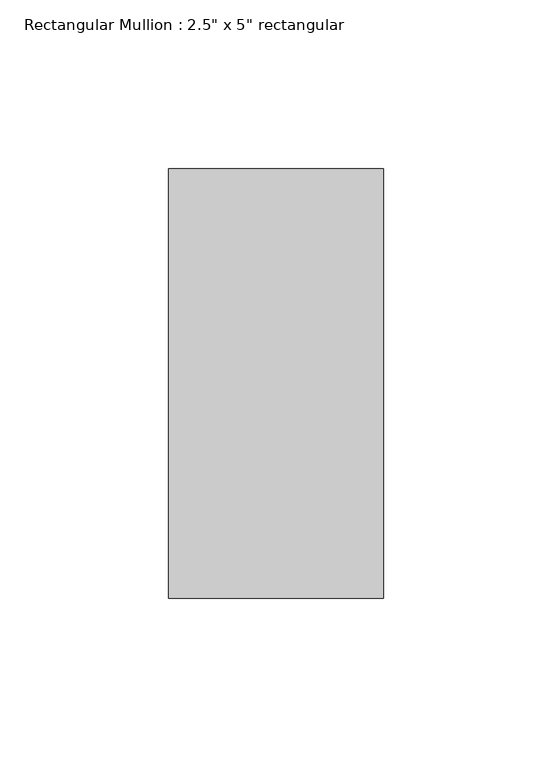
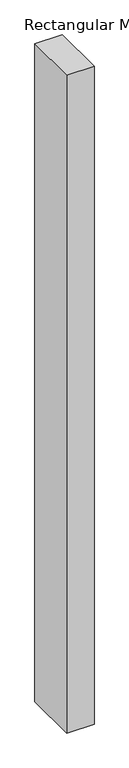
"""IFC4 building model written with IfcOpenShell, lengths in millimetres: member geometry."""

from ifc_helpers import new_model, si_unit, frame, origin, place, context, project, spatial, polyline, outline, extrude, source, transform, mapped, element, save


def member_bc7c5251(model_context):
    return source(origin(), model_context, "Body", "SweptSolid", [
        extrude(outline(polyline([(31.75, 63.5), (31.75, -63.5), (-31.75, -63.5), (-31.75, 63.5), (31.75, 63.5)])), frame((0.0, 0.0, -1608.6208916), z_axis=(0.0, 0.0, 1.0), x_axis=(1.0, 0.0, 0.0)), (0.0, 0.0, 1.0), 1608.6208916),
    ])


if __name__ == "__main__":
    model = new_model("IFC4")
    model_context = context("Model", 3, world=origin())
    ifc_project = project(units=[si_unit("LENGTHUNIT", "METRE", prefix="MILLI")], contexts=[model_context])
    site = spatial("IfcSite", under=ifc_project)
    building = spatial("IfcBuilding", under=site)
    placement = place(None, origin())
    member_shape = member_bc7c5251(model_context)
    element("IfcMember", 1, ObjectType="Rectangular Mullion : 2.5\" x 5\" rectangular", at=placement, inside=building, context=model_context, shape_type="MappedRepresentation", body=[
        mapped(member_shape, transform((0.0, 0.0, 0.0), x_axis=(1.0, 0.0, 0.0), y_axis=(0.0, 1.0, 0.0), z_axis=(0.0, 0.0, 1.0))),
    ])
    save(model, "model.ifc")

# Revit data of these elements
# Type "Rectangular Mullion : 2.5\" x 5\" rectangular"
#   built-in parameter 1007304 = 0.416667 (stored number, unit not read)
#   built-in parameter 1007301 = 0.104167 (stored number, unit not read)
#   built-in parameter 1007300 = 0.104167 (stored number, unit not read)
# Element 1 (IfcMember, "Rectangular Mullion : 2.5\" x 5\" rectangular")
#   Materials on its faces: "Aluminum"
# Materials
#   "Aluminum": class "Metal", colour RGB 247 247 247, transparency 0, Description = "Aluminum 6061", Cost = 0
